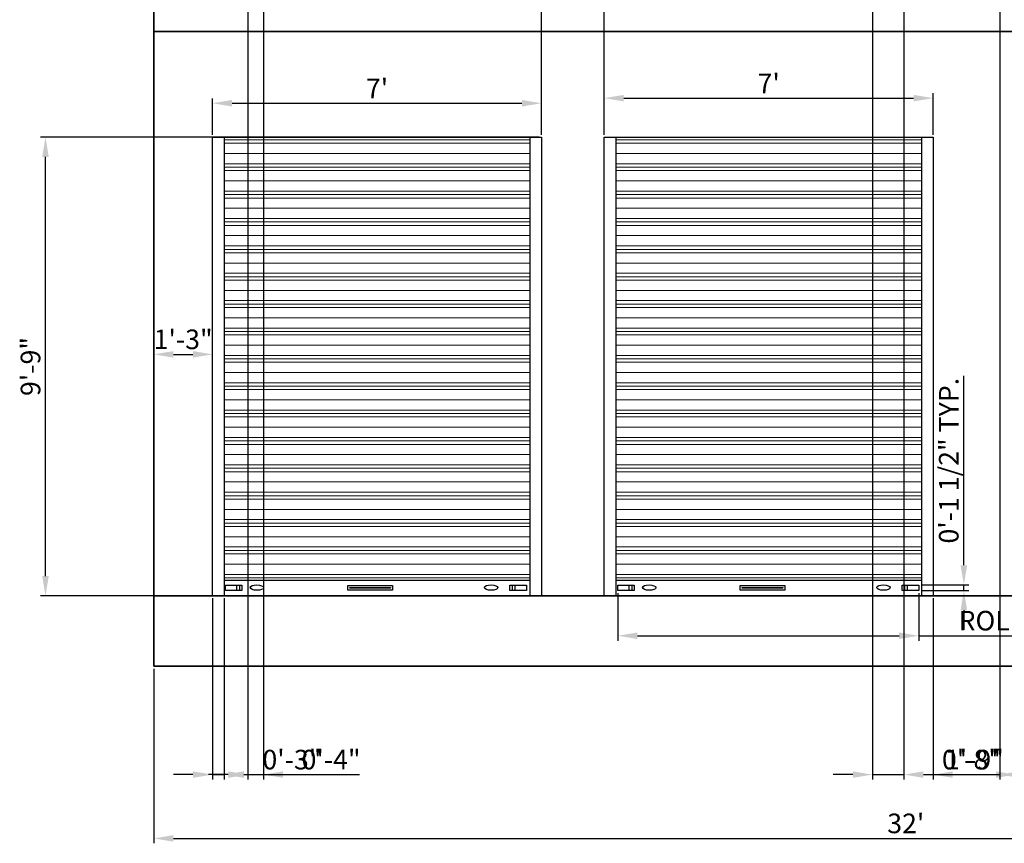
# Model space of a CAD drawing. Units: inches. Extents: x 2406 to 2953, y 1777 to 2285.
# Tile 1 of 5: x 2410 to 2661, y 1777 to 1987. Entities that reach past the tile are written whole.
import ezdxf

# ---------------------------------------------------------------- set-up
doc = ezdxf.new("R2010")
doc.units = ezdxf.units.IN
for name, color, linetype, lineweight in [('A-ANNO-DIMS', 2, 'Continuous', 18), ('A-DOOR', 3, 'Continuous', 25), ('A-ELEV', 7, 'Continuous', 35), ('A-ELEV-PATT', 253, 'Continuous', 13)]:
    doc.layers.add(name, color=color, linetype=linetype, lineweight=lineweight)
doc.styles.get("Standard").update_dxf_attribs({"font": 'arial.ttf'})
doc.dimstyles.new('ISO-25', dxfattribs={"dimtxt": 5, "dimasz": 5, "dimexe": 1.25, "dimexo": 0.625, "dimtad": 1, "dimdec": 0, "dimlunit": 3, "dimtxsty": 'Standard', "dimcen": 2.5, "dimadec": 0, "dimazin": 0, "dimtfac": 1, "dimtdec": 0, "dimtmove": 0, "dimatfit": 3, "dimfxl": 1, "dimarcsym": 0})

# ---------------------------------------------------------------- blocks, each defined once
blk = doc.blocks.new('*D2')
at = {"layer": 'A-ANNO-DIMS', "color": 0, "lineweight": -2, "transparency": 16777216}
for p, q in [((2443.83, 1821.72), (2443.83, 1777.16)), ((2827.83, 1821.72), (2827.83, 1777.16)), ((2448.83, 1778.41), (2822.83, 1778.41))]:
    blk.add_line(p, q, dxfattribs=at)
at = {"layer": 'A-ANNO-DIMS', "color": 0, "transparency": 16777216}
for points in [[(2448.83, 1779.24), (2448.83, 1777.58), (2443.83, 1778.41)], [(2822.83, 1779.24), (2822.83, 1777.58), (2827.83, 1778.41)]]:
    blk.add_solid(points, dxfattribs=at)
at = {"layer": 'Defpoints', "color": 0, "transparency": 16777216}
for p in [(2443.83, 1822.34), (2827.83, 1822.34), (2827.83, 1778.41)]:
    blk.add_point(p, dxfattribs=at)
at = {"layer": 'A-ANNO-DIMS', "color": 0, "transparency": 16777216, "insert": (2635.83, 1781.59), "char_height": 5, "attachment_point": 5}
blk.add_mtext("32'", dxfattribs=at)
blk = doc.blocks.new('*D6')
at = {"layer": 'A-ANNO-DIMS', "color": 0, "lineweight": -2, "transparency": 16777216}
for p, q in [((2458.83, 1957.97), (2458.83, 1967.27)), ((2463.83, 1966.02), (2537.83, 1966.02)), ((2542.83, 1957.97), (2542.83, 1967.27))]:
    blk.add_line(p, q, dxfattribs=at)
at = {"layer": 'A-ANNO-DIMS', "color": 0, "transparency": 16777216}
for points in [[(2463.83, 1966.85), (2463.83, 1965.18), (2458.83, 1966.02)], [(2537.83, 1966.85), (2537.83, 1965.18), (2542.83, 1966.02)]]:
    blk.add_solid(points, dxfattribs=at)
at = {"layer": 'Defpoints', "color": 0, "transparency": 16777216}
for p in [(2542.83, 1966.02), (2458.83, 1957.34), (2542.83, 1957.34)]:
    blk.add_point(p, dxfattribs=at)
at = {"layer": 'A-ANNO-DIMS', "color": 0, "transparency": 16777216, "insert": (2500.83, 1969.14), "char_height": 5, "attachment_point": 5}
blk.add_mtext("7'", dxfattribs=at)
blk = doc.blocks.new('*D15')
at = {"layer": 'A-ANNO-DIMS', "color": 0, "lineweight": -2, "transparency": 16777216}
for p, q in [((2558.83, 1957.97), (2558.83, 1968.57)), ((2642.83, 1957.97), (2642.83, 1968.57)), ((2563.83, 1967.32), (2637.83, 1967.32))]:
    blk.add_line(p, q, dxfattribs=at)
at = {"layer": 'A-ANNO-DIMS', "color": 0, "transparency": 16777216}
for points in [[(2563.83, 1968.15), (2563.83, 1966.49), (2558.83, 1967.32)], [(2637.83, 1968.15), (2637.83, 1966.49), (2642.83, 1967.32)]]:
    blk.add_solid(points, dxfattribs=at)
at = {"layer": 'Defpoints', "color": 0, "transparency": 16777216}
for p in [(2642.83, 1967.32), (2558.83, 1957.34), (2642.83, 1957.34)]:
    blk.add_point(p, dxfattribs=at)
at = {"layer": 'A-ANNO-DIMS', "color": 0, "transparency": 16777216, "insert": (2600.83, 1970.44), "char_height": 5, "attachment_point": 5}
blk.add_mtext("7'", dxfattribs=at)
blk = doc.blocks.new('*D30')
at = {"layer": 'A-ANNO-DIMS', "color": 0, "lineweight": -2, "transparency": 16777216}
for p, q in [((2443.83, 1897.51), (2443.83, 1903.19)), ((2458.83, 1894.07), (2458.83, 1903.19)), ((2448.83, 1901.94), (2453.83, 1901.94))]:
    blk.add_line(p, q, dxfattribs=at)
at = {"layer": 'A-ANNO-DIMS', "color": 0, "transparency": 16777216}
for points in [[(2448.83, 1902.77), (2448.83, 1901.11), (2443.83, 1901.94)], [(2453.83, 1902.77), (2453.83, 1901.11), (2458.83, 1901.94)]]:
    blk.add_solid(points, dxfattribs=at)
at = {"layer": 'Defpoints', "color": 0, "transparency": 16777216}
for p in [(2458.83, 1901.94), (2443.83, 1896.89), (2458.83, 1893.44)]:
    blk.add_point(p, dxfattribs=at)
at = {"layer": 'A-ANNO-DIMS', "color": 0, "transparency": 16777216, "insert": (2451.33, 1905.12), "char_height": 5, "attachment_point": 5}
blk.add_mtext('1\'-3"', dxfattribs=at)
blk = doc.blocks.new('SHUTTER-BOTTOM-BAR')
for p, q in [((1.28, 0), (0.7, 0)), ((2.93, 0), (2.93, 1.37)), ((3.56, 1.37), (3.56, 0)), ((73.32, 0), (73.32, 1.37)), ((73.89, 0), (73.32, 0)), ((73.89, 1.37), (73.89, 0))]:
    blk.add_line(p, q)
for points in [[(0, 1.37), (4.21, 1.37), (4.21, 0), (0, 0)], [(0, 1.37), (4.21, 1.37), (4.21, 0), (0, 0)], [(31.25, 1.3), (42.61, 1.3), (42.61, 0.14), (31.25, 0.14)], [(31.75, 0.8), (42.11, 0.8), (42.11, 0.64), (31.75, 0.64)], [(72.62, 1.37), (76.83, 1.37), (76.83, 0), (72.62, 0)]]:
    blk.add_lwpolyline(points, close=True)
for centre in [(8.01, 0.77), (67.82, 0.77)]:
    blk.add_ellipse(centre, major_axis=(1.71, -0.02), ratio=0.39954)
blk = doc.blocks.new('*D43')
at = {"layer": 'A-ANNO-DIMS', "color": 0, "lineweight": -2, "transparency": 16777216}
for p, q in [((2562.31, 1841.02), (2562.31, 1828.87)), ((2639.14, 1841.02), (2639.14, 1828.87)), ((2567.31, 1830.12), (2634.14, 1830.12)), ((2639.14, 1830.12), (2791.26, 1830.12))]:
    blk.add_line(p, q, dxfattribs=at)
at = {"layer": 'A-ANNO-DIMS', "color": 0, "transparency": 16777216}
for points in [[(2567.31, 1830.96), (2567.31, 1829.29), (2562.31, 1830.12)], [(2634.14, 1830.96), (2634.14, 1829.29), (2639.14, 1830.12)]]:
    blk.add_solid(points, dxfattribs=at)
at = {"layer": 'Defpoints', "color": 0, "transparency": 16777216}
for p in [(2562.31, 1841.65), (2639.14, 1841.65), (2639.14, 1830.12)]:
    blk.add_point(p, dxfattribs=at)
at = {"layer": 'A-ANNO-DIMS', "color": 0, "transparency": 16777216, "insert": (2717.7, 1833.33), "char_height": 5, "attachment_point": 5}
blk.add_mtext('ROLLING SHUTTER BOTTOM BAR 6\'-5" TYP.', dxfattribs=at)
blk = doc.blocks.new('*D44')
at = {"layer": 'A-ANNO-DIMS', "color": 0, "lineweight": -2, "transparency": 16777216}
for p, q in [((2650.66, 1848.11), (2650.66, 1896.49)), ((2639.76, 1843.11), (2651.91, 1843.11)), ((2650.66, 1841.65), (2650.66, 1843.11)), ((2639.76, 1841.65), (2651.91, 1841.65)), ((2650.66, 1836.65), (2650.66, 1831.65))]:
    blk.add_line(p, q, dxfattribs=at)
at = {"layer": 'A-ANNO-DIMS', "color": 0, "transparency": 16777216}
for points in [[(2649.83, 1848.11), (2651.5, 1848.11), (2650.66, 1843.11)], [(2649.83, 1836.65), (2651.5, 1836.65), (2650.66, 1841.65)]]:
    blk.add_solid(points, dxfattribs=at)
at = {"layer": 'Defpoints', "color": 0, "transparency": 16777216}
for p in [(2639.14, 1843.11), (2650.66, 1843.11), (2639.14, 1841.65)]:
    blk.add_point(p, dxfattribs=at)
at = {"layer": 'A-ANNO-DIMS', "color": 0, "transparency": 16777216, "insert": (2647.45, 1874.8), "char_height": 5, "attachment_point": 5, "rotation": 90}
blk.add_mtext('0\'-1 1/2" TYP.', dxfattribs=at)
blk = doc.blocks.new('*D45')
at = {"layer": 'A-ANNO-DIMS', "color": 0, "lineweight": -2, "transparency": 16777216}
for p, q in [((2673.85, 1912.9), (2673.85, 2012.41)), ((2681.47, 1912.9), (2672.6, 1912.9)), ((2673.85, 1862.91), (2673.85, 1907.9)), ((2681.47, 1857.91), (2672.6, 1857.91))]:
    blk.add_line(p, q, dxfattribs=at)
at = {"layer": 'A-ANNO-DIMS', "color": 0, "transparency": 16777216}
for points in [[(2673.01, 1907.9), (2674.68, 1907.9), (2673.85, 1912.9)], [(2673.01, 1862.91), (2674.68, 1862.91), (2673.85, 1857.91)]]:
    blk.add_solid(points, dxfattribs=at)
at = {"layer": 'Defpoints', "color": 0, "transparency": 16777216}
for p in [(2673.85, 1912.9), (2682.1, 1912.9), (2682.1, 1857.91)]:
    blk.add_point(p, dxfattribs=at)
at = {"layer": 'A-ANNO-DIMS', "color": 0, "transparency": 16777216, "insert": (2670.64, 1965.16), "char_height": 5, "attachment_point": 5, "rotation": 90}
blk.add_mtext('GATE ORNAMENT 4\'-7" TYP.', dxfattribs=at)
blk = doc.blocks.new('*D47')
at = {"layer": 'A-ANNO-DIMS', "color": 0, "lineweight": -2, "transparency": 16777216}
for p, q in [((2542.83, 1957.97), (2542.83, 2275.24)), ((2558.83, 1957.97), (2558.83, 2275.24)), ((2547.83, 2273.99), (2553.83, 2273.99))]:
    blk.add_line(p, q, dxfattribs=at)
at = {"layer": 'A-ANNO-DIMS', "color": 0, "transparency": 16777216}
for points in [[(2547.83, 2274.82), (2547.83, 2273.16), (2542.83, 2273.99)], [(2553.83, 2274.82), (2553.83, 2273.16), (2558.83, 2273.99)]]:
    blk.add_solid(points, dxfattribs=at)
at = {"layer": 'Defpoints', "color": 0, "transparency": 16777216}
for p in [(2558.83, 2273.99), (2542.83, 1957.34), (2558.83, 1957.34)]:
    blk.add_point(p, dxfattribs=at)
at = {"layer": 'A-ANNO-DIMS', "color": 0, "transparency": 16777216, "insert": (2550.83, 2277.13), "char_height": 5, "attachment_point": 5}
blk.add_mtext('1\'-4"', dxfattribs=at)
blk = doc.blocks.new('*D48')
at = {"layer": 'A-ANNO-DIMS', "color": 0, "lineweight": -2, "transparency": 16777216}
for p, q in [((2642.83, 1839.72), (2642.83, 1793.44)), ((2663.83, 1839.72), (2663.83, 1793.44)), ((2647.83, 1794.69), (2658.83, 1794.69))]:
    blk.add_line(p, q, dxfattribs=at)
at = {"layer": 'A-ANNO-DIMS', "color": 0, "transparency": 16777216}
for points in [[(2647.83, 1795.52), (2647.83, 1793.86), (2642.83, 1794.69)], [(2658.83, 1795.52), (2658.83, 1793.86), (2663.83, 1794.69)]]:
    blk.add_solid(points, dxfattribs=at)
at = {"layer": 'Defpoints', "color": 0, "transparency": 16777216}
for p in [(2642.83, 1840.34), (2663.83, 1840.34), (2663.83, 1794.69)]:
    blk.add_point(p, dxfattribs=at)
at = {"layer": 'A-ANNO-DIMS', "color": 0, "transparency": 16777216, "insert": (2653.33, 1797.87), "char_height": 5, "attachment_point": 5}
blk.add_mtext('1\'-9"', dxfattribs=at)
blk = doc.blocks.new('*D54')
at = {"layer": 'A-ANNO-DIMS', "color": 0, "lineweight": -2, "transparency": 16777216}
for p, q in [((2542.21, 1957.34), (2414.93, 1957.34)), ((2416.18, 1845.34), (2416.18, 1952.34)), ((2542.21, 1840.34), (2414.93, 1840.34))]:
    blk.add_line(p, q, dxfattribs=at)
at = {"layer": 'A-ANNO-DIMS', "color": 0, "transparency": 16777216}
for points in [[(2415.35, 1952.34), (2417.02, 1952.34), (2416.18, 1957.34)], [(2415.35, 1845.34), (2417.02, 1845.34), (2416.18, 1840.34)]]:
    blk.add_solid(points, dxfattribs=at)
at = {"layer": 'Defpoints', "color": 0, "transparency": 16777216}
for p in [(2416.18, 1957.34), (2542.83, 1957.34), (2542.83, 1840.34)]:
    blk.add_point(p, dxfattribs=at)
at = {"layer": 'A-ANNO-DIMS', "color": 0, "transparency": 16777216, "insert": (2413.01, 1898.84), "char_height": 5, "attachment_point": 5, "rotation": 90}
blk.add_mtext('9\'-9"', dxfattribs=at)
blk = doc.blocks.new('*D55')
at = {"layer": 'A-ANNO-DIMS', "color": 0, "lineweight": -2, "transparency": 16777216}
for p, q in [((2458.83, 1839.72), (2458.83, 1793.44)), ((2461.83, 1839.72), (2461.83, 1793.44)), ((2453.83, 1794.69), (2448.83, 1794.69)), ((2458.83, 1794.69), (2461.83, 1794.69)), ((2466.83, 1794.69), (2486.37, 1794.69))]:
    blk.add_line(p, q, dxfattribs=at)
at = {"layer": 'A-ANNO-DIMS', "color": 0, "transparency": 16777216}
for points in [[(2453.83, 1795.52), (2453.83, 1793.86), (2458.83, 1794.69)], [(2466.83, 1795.52), (2466.83, 1793.86), (2461.83, 1794.69)]]:
    blk.add_solid(points, dxfattribs=at)
at = {"layer": 'Defpoints', "color": 0, "transparency": 16777216}
for p in [(2458.83, 1840.34), (2461.83, 1840.34), (2461.83, 1794.69)]:
    blk.add_point(p, dxfattribs=at)
at = {"layer": 'A-ANNO-DIMS', "color": 0, "transparency": 16777216, "insert": (2479.1, 1797.87), "char_height": 5, "attachment_point": 5}
blk.add_mtext('0\'-3"', dxfattribs=at)
blk = doc.blocks.new('*D62')
at = {"layer": 'A-ANNO-DIMS', "color": 0, "lineweight": -2, "transparency": 16777216}
for p, q in [((2467.83, 2037.72), (2467.83, 1793.44)), ((2471.83, 2037.72), (2471.83, 1793.44)), ((2462.83, 1794.69), (2457.83, 1794.69)), ((2467.83, 1794.69), (2471.83, 1794.69)), ((2476.83, 1794.69), (2496.37, 1794.69))]:
    blk.add_line(p, q, dxfattribs=at)
at = {"layer": 'A-ANNO-DIMS', "color": 0, "transparency": 16777216}
for points in [[(2462.83, 1795.52), (2462.83, 1793.86), (2467.83, 1794.69)], [(2476.83, 1795.52), (2476.83, 1793.86), (2471.83, 1794.69)]]:
    blk.add_solid(points, dxfattribs=at)
at = {"layer": 'Defpoints', "color": 0, "transparency": 16777216}
for p in [(2467.83, 2038.34), (2471.83, 2038.34), (2471.83, 1794.69)]:
    blk.add_point(p, dxfattribs=at)
at = {"layer": 'A-ANNO-DIMS', "color": 0, "transparency": 16777216, "insert": (2489.1, 1797.87), "char_height": 5, "attachment_point": 5}
blk.add_mtext('0\'-4"', dxfattribs=at)
blk = doc.blocks.new('*D64')
at = {"layer": 'A-ANNO-DIMS', "color": 0, "lineweight": -2, "transparency": 16777216}
for p, q in [((2659.83, 2103.72), (2659.83, 1793.44)), ((2671.83, 2089.72), (2671.83, 1793.44)), ((2664.83, 1794.69), (2666.83, 1794.69)), ((2671.83, 1794.69), (2690.9, 1794.69))]:
    blk.add_line(p, q, dxfattribs=at)
at = {"layer": 'A-ANNO-DIMS', "color": 0, "transparency": 16777216}
for points in [[(2664.83, 1795.52), (2664.83, 1793.86), (2659.83, 1794.69)], [(2666.83, 1795.52), (2666.83, 1793.86), (2671.83, 1794.69)]]:
    blk.add_solid(points, dxfattribs=at)
at = {"layer": 'Defpoints', "color": 0, "transparency": 16777216}
for p in [(2659.83, 2104.34), (2671.83, 2090.34), (2671.83, 1794.69)]:
    blk.add_point(p, dxfattribs=at)
at = {"layer": 'A-ANNO-DIMS', "color": 0, "transparency": 16777216, "insert": (2683.87, 1797.87), "char_height": 5, "attachment_point": 5}
blk.add_mtext('1\'-0"', dxfattribs=at)
blk = doc.blocks.new('*D76')
at = {"layer": 'A-ANNO-DIMS', "color": 0, "lineweight": -2, "transparency": 16777216}
for p, q in [((2627.33, 2127.72), (2627.33, 1793.44)), ((2635.33, 2127.72), (2635.33, 1793.44)), ((2622.33, 1794.69), (2617.33, 1794.69)), ((2627.33, 1794.69), (2635.33, 1794.69)), ((2640.33, 1794.69), (2659.87, 1794.69))]:
    blk.add_line(p, q, dxfattribs=at)
at = {"layer": 'A-ANNO-DIMS', "color": 0, "transparency": 16777216}
for points in [[(2622.33, 1795.52), (2622.33, 1793.86), (2627.33, 1794.69)], [(2640.33, 1795.52), (2640.33, 1793.86), (2635.33, 1794.69)]]:
    blk.add_solid(points, dxfattribs=at)
at = {"layer": 'Defpoints', "color": 0, "transparency": 16777216}
for p in [(2627.33, 2128.34), (2635.33, 2128.34), (2635.33, 1794.69)]:
    blk.add_point(p, dxfattribs=at)
at = {"layer": 'A-ANNO-DIMS', "color": 0, "transparency": 16777216, "insert": (2652.6, 1797.87), "char_height": 5, "attachment_point": 5}
blk.add_mtext('0\'-8"', dxfattribs=at)

msp = doc.modelspace()

# ---------------------------------------------------------------- hatches: boundary and pattern name
at = {"layer": 'A-ELEV-PATT'}
h = msp.add_hatch(dxfattribs=at)
h.set_pattern_fill('PLASTI', color=256, scale=1.1)
h.paths.add_polyline_path([(2539.83, 1957.34), (2461.83, 1957.34), (2461.83, 1844.34), (2539.83, 1844.34)])
h.paths.add_polyline_path([(2639.83, 1957.34), (2561.83, 1957.34), (2561.83, 1844.34), (2639.83, 1844.34)])

# ---------------------------------------------------------------- linework, layer by layer
at = {"layer": 'A-DOOR'}
for p, q in [((2461.83, 1957.34), (2461.83, 1840.34)), ((2539.83, 1957.34), (2539.83, 1840.34)), ((2561.83, 1957.34), (2561.83, 1840.34)), ((2639.83, 1957.34), (2639.83, 1840.34)), ((2461.83, 1844.34), (2539.83, 1844.34)), ((2561.83, 1844.34), (2639.83, 1844.34))]:
    msp.add_line(p, q, dxfattribs=at)
for points in [[(2458.83, 1840.34), (2458.83, 1957.34), (2542.83, 1957.34), (2542.83, 1840.34)], [(2558.83, 1840.34), (2558.83, 1957.34), (2642.83, 1957.34), (2642.83, 1840.34)]]:
    msp.add_lwpolyline(points, dxfattribs=at)
at = {"layer": 'A-ELEV'}
for p, q in [((2443.83, 2182.34), (2443.83, 1822.34)), ((2443.83, 1984.34), (2827.83, 1984.34)), ((2443.83, 1840.34), (2827.83, 1840.34)), ((2443.83, 1822.34), (2827.83, 1822.34))]:
    msp.add_line(p, q, dxfattribs=at)

# ---------------------------------------------------------------- block references
at = {"layer": 'A-DOOR'}
for p in [(2462.14, 1841.65), (2562.31, 1841.65)]:
    msp.add_blockref('SHUTTER-BOTTOM-BAR', p, dxfattribs=at)

# ---------------------------------------------------------------- dimensions: what is measured, and where the dimension line sits
at = {"layer": 'A-ANNO-DIMS'}
for base, p1, p2, override, picture, middle in [((2558.83, 2273.99), (2542.83, 1957.34), (2558.83, 1957.34), {"dimdec": 1, "dimlfac": 1, "dimrnd": 0, "dimzin": 1, "dimdsep": 46, "dimlunit": 4, "dimfrac": 2}, '*D47', (2550.83, 2277.13)), ((2635.33, 1794.69), (2627.33, 2128.34), (2635.33, 2128.34), {"dimdec": 1, "dimlfac": 1, "dimrnd": 0, "dimzin": 1, "dimdsep": 46, "dimlunit": 4, "dimfrac": 2}, '*D76', (2652.6, 1797.87)), ((2671.83, 1794.69), (2659.83, 2104.34), (2671.83, 2090.34), {"dimdec": 1, "dimlfac": 1, "dimrnd": 0, "dimzin": 1, "dimdsep": 46, "dimlunit": 4, "dimfrac": 2}, '*D64', (2683.87, 1797.87)), ((2471.83, 1794.69), (2467.83, 2038.34), (2471.83, 2038.34), {"dimdec": 1, "dimlfac": 1, "dimrnd": 0, "dimzin": 1, "dimdsep": 46, "dimlunit": 4, "dimfrac": 2}, '*D62', (2489.1, 1797.87)), ((2642.83, 1967.32), (2558.83, 1957.34), (2642.83, 1957.34), {"dimclrd": 0, "dimclre": 0, "dimclrt": 0}, '*D15', (2600.83, 1970.44)), ((2458.83, 1901.94), (2443.83, 1896.89), (2458.83, 1893.44), {"dimclrd": 0, "dimclre": 0, "dimclrt": 0}, '*D30', (2451.33, 1905.12)), ((2461.83, 1794.69), (2458.83, 1840.34), (2461.83, 1840.34), {"dimdec": 1, "dimlfac": 1, "dimrnd": 0, "dimzin": 1, "dimdsep": 46, "dimlunit": 4, "dimfrac": 2}, '*D55', (2479.1, 1797.87)), ((2663.83, 1794.69), (2642.83, 1840.34), (2663.83, 1840.34), {"dimdec": 1, "dimlfac": 1, "dimrnd": 0, "dimzin": 1, "dimdsep": 46, "dimlunit": 4, "dimfrac": 2}, '*D48', (2653.33, 1797.87))]:
    dim = msp.add_linear_dim(base=base, p1=p1, p2=p2, dimstyle='ISO-25', override=override, dxfattribs=at)
    dim.commit()
    dim.dimension.update_dxf_attribs({"geometry": picture, "text_midpoint": middle})
for base, p1, p2, text, picture, middle in [((2673.85, 1912.9), (2682.1, 1857.91), (2682.1, 1912.9), 'GATE ORNAMENT <> TYP.', '*D45', (2670.64, 1965.16)), ((2650.66, 1843.11), (2639.14, 1841.65), (2639.14, 1843.11), '<> TYP.', '*D44', (2647.45, 1874.8))]:
    dim = msp.add_linear_dim(base=base, p1=p1, p2=p2, angle=90, text=text, dimstyle='ISO-25', override={"dimdec": 1, "dimrnd": 0, "dimzin": 1, "dimlunit": 4, "dimfrac": 2}, dxfattribs=at)
    dim.commit()
    dim.dimension.update_dxf_attribs({"geometry": picture, "text_midpoint": middle})
for base, p1, p2, picture, middle in [((2542.83, 1966.02), (2458.83, 1957.34), (2542.83, 1957.34), '*D6', (2500.83, 1966.02)), ((2827.83, 1778.41), (2443.83, 1822.34), (2827.83, 1822.34), '*D2', (2635.83, 1778.41))]:
    dim = msp.add_linear_dim(base=base, p1=p1, p2=p2, dimstyle='ISO-25', override={"dimclrd": 0, "dimclre": 0, "dimclrt": 0}, dxfattribs=at)
    dim.commit()
    dim.dimension.update_dxf_attribs({"geometry": picture, "text_midpoint": middle, "dimtype": 160})
dim = msp.add_linear_dim(base=(2416.18, 1957.34), p1=(2542.83, 1840.34), p2=(2542.83, 1957.34), angle=90, dimstyle='ISO-25', override={"dimdec": 1, "dimlfac": 1, "dimrnd": 0, "dimzin": 1, "dimdsep": 46, "dimlunit": 4, "dimfrac": 2}, dxfattribs=at)
dim.commit()
dim.dimension.update_dxf_attribs({"geometry": '*D54', "text_midpoint": (2413.01, 1898.84)})
dim = msp.add_linear_dim(base=(2639.14, 1830.12), p1=(2562.31, 1841.65), p2=(2639.14, 1841.65), text='ROLLING SHUTTER BOTTOM BAR <> TYP.', dimstyle='ISO-25', override={"dimdec": 1, "dimrnd": 0, "dimzin": 1, "dimlunit": 4, "dimfrac": 2}, dxfattribs=at)
dim.commit()
dim.dimension.update_dxf_attribs({"geometry": '*D43', "text_midpoint": (2717.7, 1833.33)})

doc.saveas('drawing.dxf')
